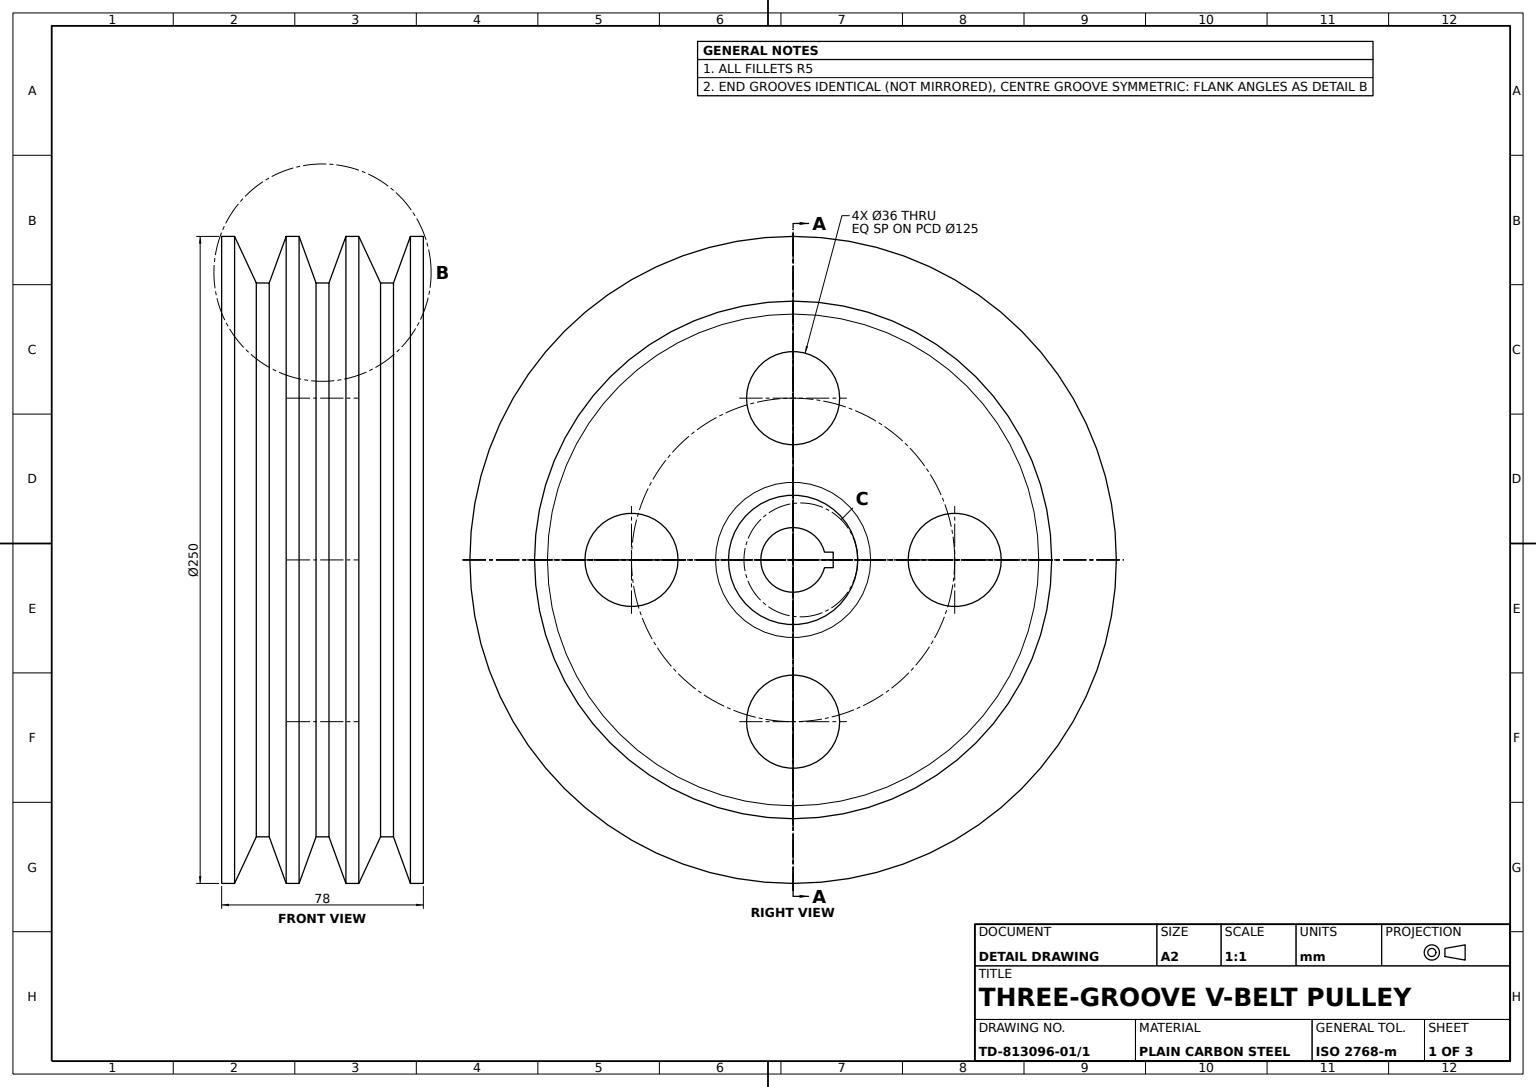
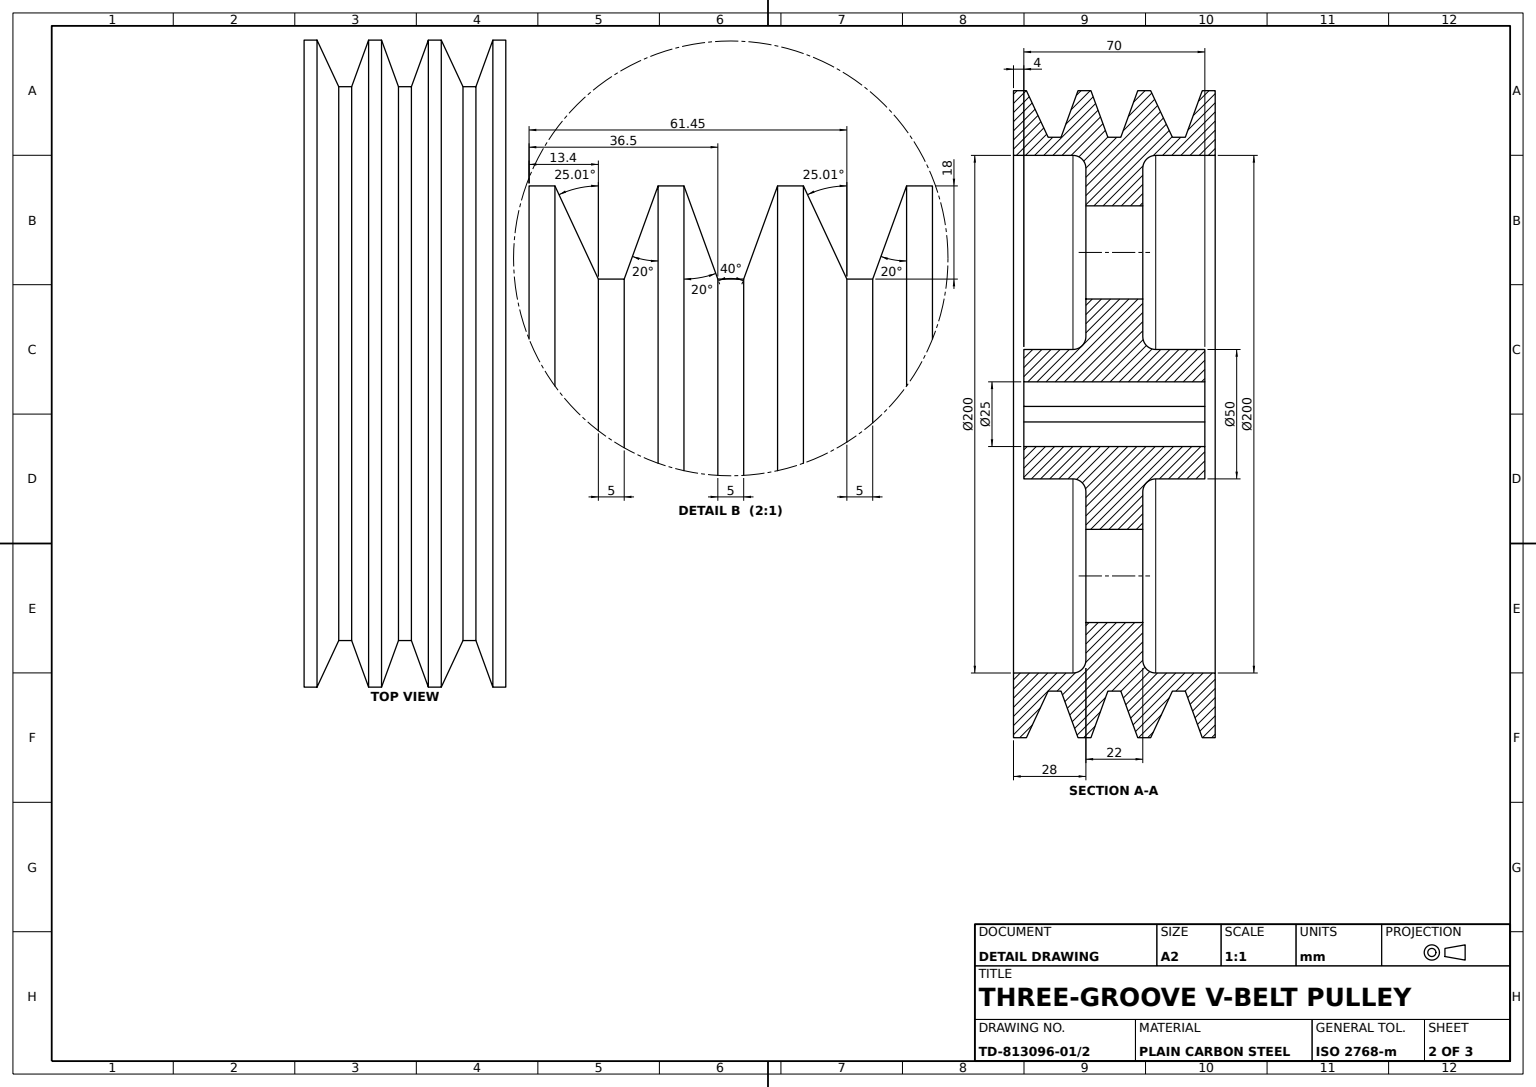
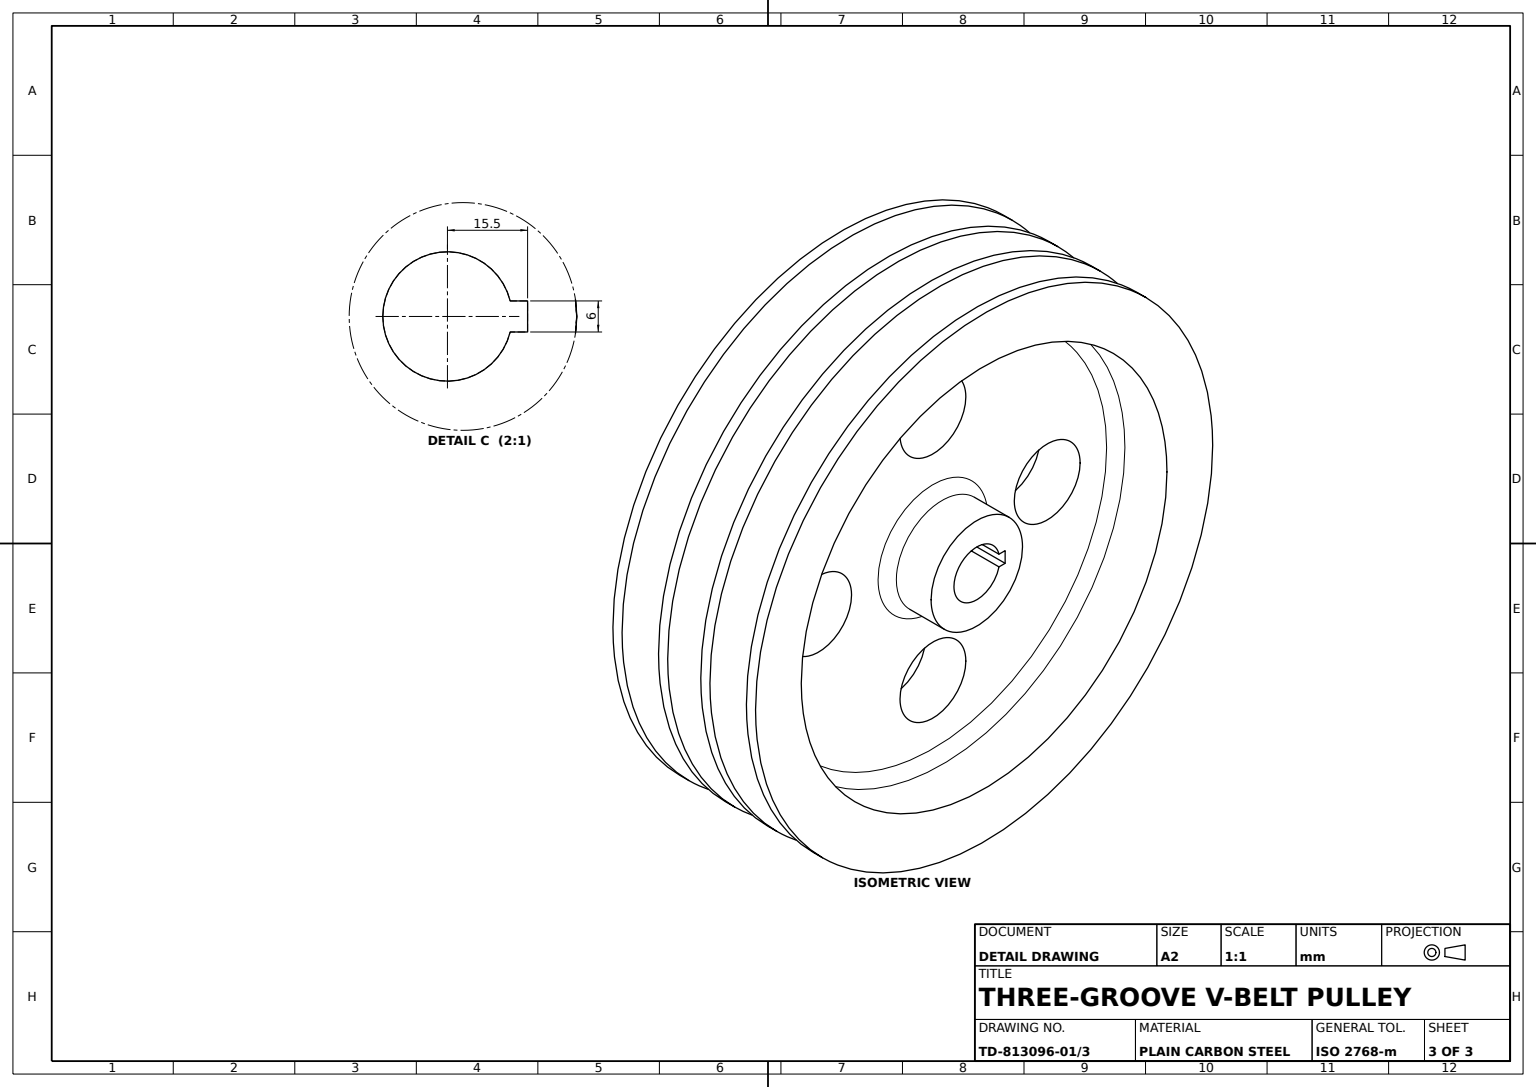
from build123d import *

# Parameters (mm, degrees)
EDGE_FILLET_R5_A_R           = 5
EDGE_FILLET_R5_B_R           = 5
EDGE_FILLET_R5_C_R           = 5
KEYWAY_6X6_DEPTH             = 80
LIGHTENING_HOLES_SKETCH_R    = 18
LIGHTENING_HOLES_4X_36_DEPTH = 45


with BuildPart() as part:
    # Pulley Profile Sketch → Pulley Body Revolve (revolve)
    with BuildSketch(Plane.XY, mode=Mode.PRIVATE) as pulley_body_revolve_sk:
        Polygon((-35, 12.5), (35, 12.5), (35, 25), (11, 25), (11, 100), (39, 100), (39, 125), (34, 125), (27.448535783, 107), (22.448535783, 107), (14.051464217, 125), (9.051464217, 125), (2.5, 107), (-2.5, 107), (-9.051464217, 125), (-14.051464217, 125), (-20.602928434, 107), (-25.602928434, 107), (-34, 125), (-39, 125), (-39, 100), (-11, 100), (-11, 25), (-35, 25), align=None)
    revolve(pulley_body_revolve_sk.sketch.rotate(Axis((-52.075788227, 0, 0), (1, 0, 0)), 90), axis=Axis((-52.075788227, 0, 0), (1, 0, 0)))

    # Edge Fillet R5 A
    edge_fillet_r5_a_edges = [part.edges().sort_by_distance(p)[0] for p in [
        (11, 0, -100),
    ]]
    fillet(edge_fillet_r5_a_edges, radius=EDGE_FILLET_R5_A_R)

    # Edge Fillet R5 B
    edge_fillet_r5_b_edges = [part.edges().sort_by_distance(p)[0] for p in [
        (11, 0, -25),
    ]]
    fillet(edge_fillet_r5_b_edges, radius=EDGE_FILLET_R5_B_R)

    # Edge Fillet R5 C
    edge_fillet_r5_c_edges = [part.edges().sort_by_distance(p)[0] for p in [
        (-11, 0, -25),
        (-11, 0, -100),
    ]]
    fillet(edge_fillet_r5_c_edges, radius=EDGE_FILLET_R5_C_R)

    # Keyway Sketch → Keyway 6x6 (cut)
    with BuildSketch(Plane(origin=(35, 0, 0), x_dir=(0, 0, -1), z_dir=(1, 0, 0))):
        with BuildLine():
            Line((12.1346611, 3), (15.5, 3))
            Line((15.5, 3), (15.5, -3))
            Line((15.5, -3), (12.1346611, -3))
            ThreePointArc((12.1346611, -3), (12.5, 0), (12.1346611, 3))
        make_face()
    extrude(amount=-KEYWAY_6X6_DEPTH, mode=Mode.SUBTRACT)

    # Lightening Holes Sketch → Lightening Holes 4xØ36 (cut, symmetric)
    with BuildSketch(Plane(origin=(11, 0, 0), x_dir=(0, 0, -1), z_dir=(1, 0, 0))):
        with Locations((0, 62.5)):
            Circle(LIGHTENING_HOLES_SKETCH_R)
        with Locations((62.5, 0)):
            Circle(LIGHTENING_HOLES_SKETCH_R)
        with Locations((0, -62.5)):
            Circle(LIGHTENING_HOLES_SKETCH_R)
        with Locations((-62.5, 0)):
            Circle(LIGHTENING_HOLES_SKETCH_R)
    extrude(amount=LIGHTENING_HOLES_4X_36_DEPTH, both=True, mode=Mode.SUBTRACT)


solid = part.part
